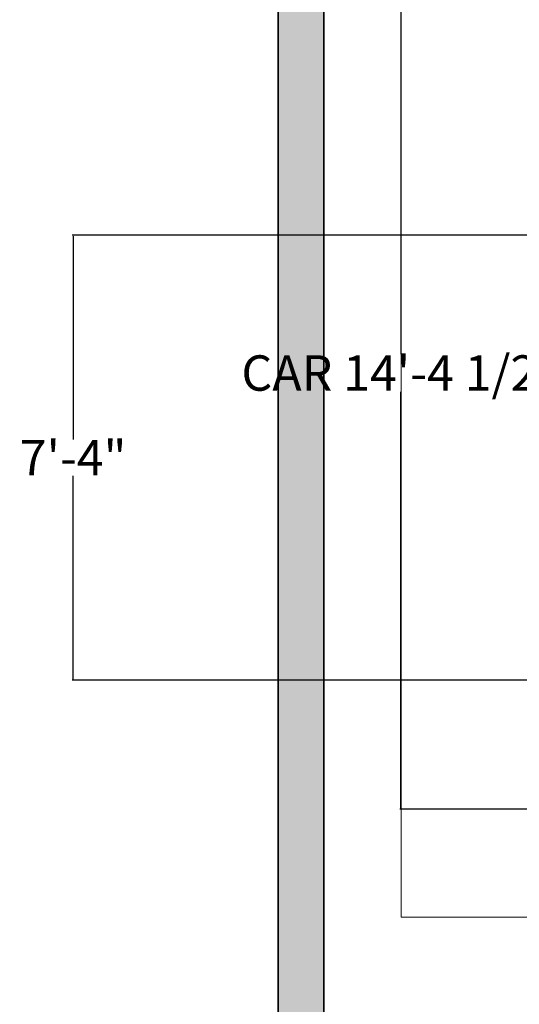
# Model space of a CAD drawing. Units: inches. Extents: x 1319 to 2030, y 219 to 1069.
# Tile 2 of 28: x 1319 to 1417, y 320 to 515. Entities that reach past the tile are written whole.
import ezdxf

# ---------------------------------------------------------------- set-up
doc = ezdxf.new("R2010")
doc.units = ezdxf.units.IN
doc.header["$MEASUREMENT"] = 0
for name, color, linetype, lineweight in [('A-ANNO-DIMS', 2, 'Continuous', 18), ('A-FLOR', 8, 'Continuous', 18), ('A-WALL-PATT', 252, 'Continuous', 13), ('C-PROP', 7, 'Continuous', 35), ('walls', 250, 'Continuous', 35)]:
    doc.layers.add(name, color=color, linetype=linetype, lineweight=lineweight)
doc.styles.get("Standard").update_dxf_attribs({"font": 'arial.ttf'})
doc.dimstyles.get("Standard").update_dxf_attribs({"dimtxt": 7, "dimasz": 0.18, "dimexe": 0.18, "dimexo": 0.0625, "dimgap": 0.09, "dimtad": 0, "dimtih": 1, "dimtoh": 1, "dimzin": 0, "dimdsep": 46, "dimlunit": 3, "dimtxsty": 'Standard', "dimcen": 0.09, "dimadec": 0, "dimazin": 0, "dimtfac": 1, "dimtofl": 0, "dimtmove": 0, "dimatfit": 3, "dimfxl": 1, "dimtolj": 1, "dimtzin": 0, "dimarcsym": 0})

# ---------------------------------------------------------------- blocks, each defined once
blk = doc.blocks.new('*D56')
at = {"layer": 'A-ANNO-DIMS', "color": 0, "lineweight": -2, "transparency": 16777216}
for p, q in [((1419.85, 531.2), (1393.86, 531.2)), ((1394.04, 531.02), (1394.04, 448.68)), ((1394.04, 358.92), (1394.04, 441.26)), ((1419.85, 358.74), (1393.86, 358.74))]:
    blk.add_line(p, q, dxfattribs=at)
at = {"layer": 'A-ANNO-DIMS', "color": 0, "transparency": 16777216}
for points in [[(1394.01, 531.02), (1394.07, 531.02), (1394.04, 531.2)], [(1394.01, 358.92), (1394.07, 358.92), (1394.04, 358.74)]]:
    blk.add_solid(points, dxfattribs=at)
at = {"layer": 'Defpoints', "color": 0, "transparency": 16777216}
for p in [(1419.91, 531.2), (1394.04, 358.74), (1419.91, 358.74)]:
    blk.add_point(p, dxfattribs=at)
at = {"layer": 'A-ANNO-DIMS', "color": 0, "transparency": 16777216, "insert": (1394.04, 444.97), "char_height": 7, "attachment_point": 5}
blk.add_mtext('\\A1;CAR 14\'-4 1/2"', dxfattribs=at)
blk = doc.blocks.new('*D65')
at = {"layer": 'A-ANNO-DIMS', "color": 0, "lineweight": -2, "transparency": 16777216}
for p, q in [((1648.280254, 472.227245), (1329.112754, 472.227245)), ((1329.292754, 472.047245), (1329.292754, 431.817245)), ((1329.292754, 384.407245), (1329.292754, 424.637245)), ((1648.280254, 384.227245), (1329.112754, 384.227245))]:
    blk.add_line(p, q, dxfattribs=at)
at = {"layer": 'A-ANNO-DIMS', "color": 0, "transparency": 16777216}
for points in [[(1329.262754, 472.047245), (1329.322754, 472.047245), (1329.292754, 472.227245)], [(1329.262754, 384.407245), (1329.322754, 384.407245), (1329.292754, 384.227245)]]:
    blk.add_solid(points, dxfattribs=at)
at = {"layer": 'Defpoints', "color": 0, "transparency": 16777216}
for p in [(1329.292754, 472.227245), (1648.342754, 472.227245), (1648.342754, 384.227245)]:
    blk.add_point(p, dxfattribs=at)
at = {"layer": 'A-ANNO-DIMS', "color": 0, "transparency": 16777216, "insert": (1329.292754, 428.227245), "char_height": 7, "attachment_point": 5}
blk.add_mtext('\\A1;7\'-4"', dxfattribs=at)

msp = doc.modelspace()

# ---------------------------------------------------------------- hatches: boundary and pattern name
at = {"layer": 'A-WALL-PATT'}
h = msp.add_hatch(color=256, dxfattribs=at)
h.dxf.hatch_style = 1
h.paths.add_polyline_path([(1378.843, 946.227), (1960.843, 946.227), (1960.843, 860.616), (1922.194, 860.616), (1922.194, 851.616), (1960.843, 851.616), (1960.843, 304.227), (1578.343, 304.227), (1578.343, 295.227), (1969.843, 295.227), (1969.843, 955.227), (1369.843, 955.227), (1369.843, 295.227), (1378.843, 295.227)])

# ---------------------------------------------------------------- linework, layer by layer
at = {"layer": 'A-FLOR'}
for p, q in [((1394.092, 567.372), (1394.092, 337.406)), ((1394.092, 337.406), (1817.431, 337.406))]:
    msp.add_line(p, q, dxfattribs=at)
at = {"layer": 'C-PROP'}
msp.add_line((1369.843, 295.227), (1369.843, 955.227), dxfattribs=at)
at = {"layer": 'walls'}
msp.add_line((1378.843, 295.227), (1378.843, 946.227), dxfattribs=at)

# ---------------------------------------------------------------- dimensions: what is measured, and where the dimension line sits
at = {"layer": 'A-ANNO-DIMS'}
dim = msp.add_linear_dim(base=(1394.045, 358.738), p1=(1419.914, 531.201), p2=(1419.914, 358.738), angle=270, text='CAR <>', dimstyle='Standard', override={"dimdec": 1, "dimlfac": 1, "dimrnd": 0, "dimzin": 1, "dimdsep": 46, "dimlunit": 4, "dimfrac": 2}, dxfattribs=at)
dim.commit()
dim.dimension.update_dxf_attribs({"geometry": '*D56', "text_midpoint": (1394.045, 444.969)})
dim = msp.add_linear_dim(base=(1329.293, 472.227), p1=(1648.343, 384.227), p2=(1648.343, 472.227), angle=90, dimstyle='Standard', override={"dimdec": 1, "dimlfac": 1, "dimrnd": 0, "dimzin": 1, "dimdsep": 46, "dimlunit": 4, "dimfrac": 2}, dxfattribs=at)
dim.commit()
dim.dimension.update_dxf_attribs({"geometry": '*D65', "text_midpoint": (1329.293, 428.227)})

doc.saveas('drawing.dxf')
